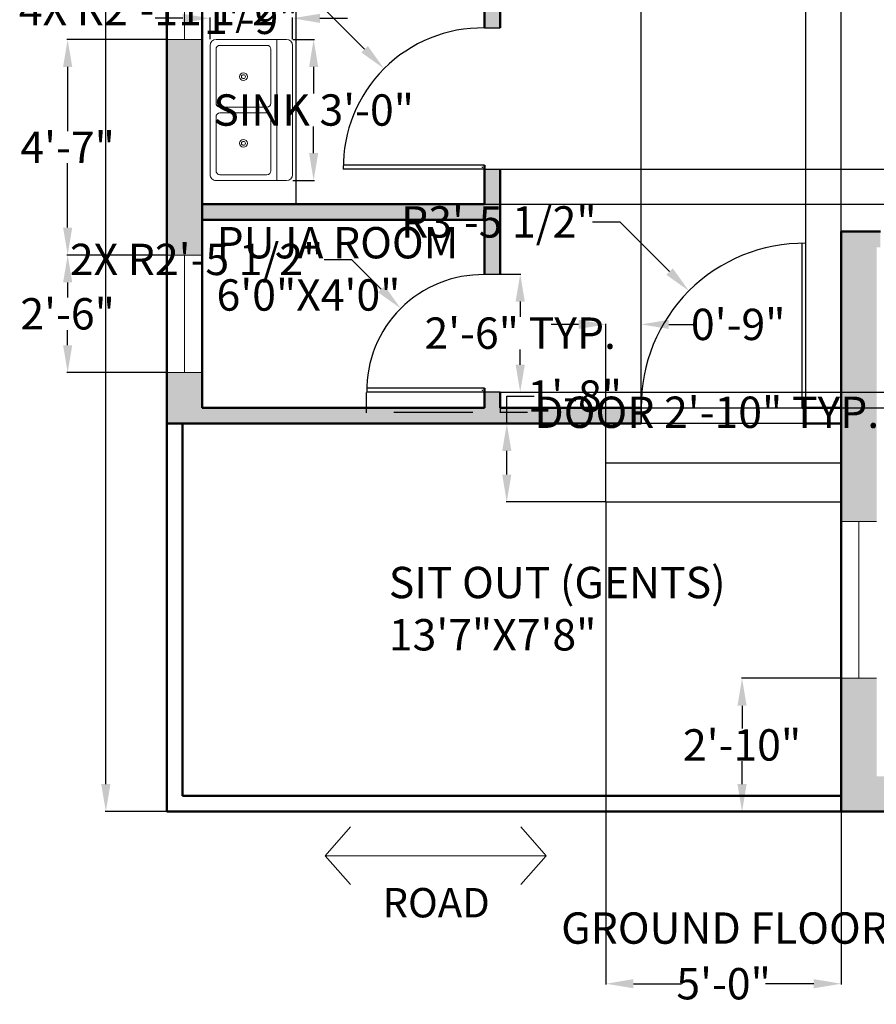
# Model space of a CAD drawing. Units: inches. Extents: x 808573 to 809030, y 884276 to 884799.
# Tile 1 of 4: x 808582 to 808801, y 884282 to 884534. Entities that reach past the tile are written whole.
import ezdxf

# ---------------------------------------------------------------- set-up
doc = ezdxf.new("R2010")
doc.units = ezdxf.units.IN
doc.header["$MEASUREMENT"] = 0
for name, color, linetype, lineweight in [('A-ANNO-DIMS', 2, 'Continuous', 18), ('A-ANNO-SYMB', 7, 'Continuous', 18), ('A-ANNO-TEXT', 7, 'Continuous', 25), ('A-AREA-IDEN', 7, 'Continuous', 25), ('A-DOOR', 3, 'Continuous', 25), ('A-FLOR-CASE', 9, 'Continuous', 25), ('A-FLOR-FIXT', 9, 'Continuous', 18), ('A-FLOR-STRS', 7, 'Continuous', 25), ('A-GLAZ', 4, 'Continuous', 18), ('A-WALL', 7, 'Continuous', 50)]:
    doc.layers.add(name, color=color, linetype=linetype, lineweight=lineweight)
doc.layers.add('A-WALL-PATT', color=251, linetype='Continuous', lineweight=13, true_color=0x636466)
doc.styles.get("Standard").update_dxf_attribs({"font": 'arial.ttf'})
doc.dimstyles.get("Standard").update_dxf_attribs({"dimtxt": 8, "dimasz": 7, "dimexe": 0.18, "dimexo": 0.0625, "dimgap": 0.09, "dimtad": 0, "dimtih": 1, "dimtoh": 1, "dimdec": 0, "dimzin": 0, "dimdsep": 46, "dimlunit": 3, "dimtxsty": 'Standard', "dimcen": 0.09, "dimadec": 0, "dimazin": 0, "dimtfac": 1, "dimtdec": 0, "dimtofl": 0, "dimtmove": 0, "dimatfit": 3, "dimfxl": 1, "dimtolj": 1, "dimtzin": 0, "dimarcsym": 0})

# ---------------------------------------------------------------- blocks, each defined once
blk = doc.blocks.new('Sink-double - 36 in top')
for p, q in [((-18, -4), (18, -4)), ((-0.75, -18.5), (-0.75, -6.5)), ((0.75, -6.5), (0.75, -18.5))]:
    blk.add_line(p, q)
for points in [[(-16.5, 0), (16.5, 0)], [(-18, -19.5), (-18, -1.5)], [(18, -1.5), (18, -19.5)], [(-16.5, -18.5), (-16.5, -6.5)], [(-15.5, -5.5), (-1.75, -5.5)], [(1.75, -5.5), (15.5, -5.5)], [(16.5, -6.5), (16.5, -18.5)], [(-1.75, -19.5), (-15.5, -19.5)], [(15.5, -19.5), (1.75, -19.5)], [(16.5, -21), (-16.5, -21)]]:
    blk.add_lwpolyline(points)
for centre, radius in [((-8.5, -12.5), 1), ((-8.5, -12.5), 0.5), ((8.5, -12.5), 1), ((8.5, -12.5), 0.5)]:
    blk.add_circle(centre, radius)
for centre, radius, start, end in [((-16.5, -1.5), 1.5, 90, 180), ((16.5, -1.5), 1.5, 0, 90), ((-15.5, -6.5), 1, 90, 180), ((-1.75, -6.5), 1, 0, 90), ((1.75, -6.5), 1, 90, 180), ((15.5, -6.5), 1, 0, 90), ((-16.5, -19.5), 1.5, 180, 270), ((-15.5, -18.5), 1, 180, 270), ((-1.75, -18.5), 1, 270, 0), ((1.75, -18.5), 1, 180, 270), ((15.5, -18.5), 1, 270, 0), ((16.5, -19.5), 1.5, 270, 0)]:
    blk.add_arc(centre, radius, start, end)
blk = doc.blocks.new('*D7')
at = {"layer": 'A-ANNO-DIMS', "color": 0, "lineweight": -2, "transparency": 16777216}
for p, q in [((808619.57, 884751.64), (808603.89, 884751.64)), ((808604.07, 884744.64), (808604.07, 884545.82)), ((808604.07, 884338.64), (808604.07, 884537.46)), ((808619.57, 884331.64), (808603.89, 884331.64))]:
    blk.add_line(p, q, dxfattribs=at)
at = {"layer": 'A-ANNO-DIMS', "color": 0, "transparency": 16777216}
for points in [[(808602.9, 884744.64), (808605.23, 884744.64), (808604.07, 884751.64)], [(808602.9, 884338.64), (808605.23, 884338.64), (808604.07, 884331.64)]]:
    blk.add_solid(points, dxfattribs=at)
at = {"layer": 'Defpoints', "color": 0, "transparency": 16777216}
for p in [(808619.63, 884751.64), (808604.07, 884331.64), (808619.63, 884331.64)]:
    blk.add_point(p, dxfattribs=at)
at = {"layer": 'A-ANNO-DIMS', "color": 0, "transparency": 16777216, "insert": (808604.07, 884541.64), "char_height": 8, "attachment_point": 5}
blk.add_mtext("\\A1;35'", dxfattribs=at)
blk = doc.blocks.new('DOOR-SWING-36IN')
for p, q in [((0, 0), (0, 36)), ((1, 0), (1, 36)), ((0, 0), (0, -4)), ((36, 0), (36, -4))]:
    blk.add_line(p, q)
blk.add_arc((0.5, 0.5), 35.5, 359.1931, 90.8069)
blk = doc.blocks.new('DOOR-SWING-30IN')
for p, q in [((0, 30), (-4, 30)), ((-4, 1), (-34, 1)), ((-4, 0), (-34, 0)), ((0, 0), (-4, 0))]:
    blk.add_line(p, q)
blk.add_arc((-4.5, 0.5), 29.5, 89.029, 180.971)
blk = doc.blocks.new('WIN-40IN')
for p, q in [((0, 0), (9, 0)), ((4.5, 0), (4.5, -40)), ((0, -40), (9, -40))]:
    blk.add_line(p, q)
blk = doc.blocks.new('WIN-36IN')
for p, q in [((0, 0), (-9, 0)), ((-4.5, 0), (-4.5, -36)), ((0, -36), (-9, -36))]:
    blk.add_line(p, q)
blk = doc.blocks.new('*D21')
at = {"layer": 'A-ANNO-DIMS', "color": 0, "lineweight": -2, "transparency": 16777216}
for p, q in [((808670.49, 884438.58), (808670.49, 884433.34)), ((808704.63, 884438.58), (808704.63, 884433.34)), ((808677.49, 884433.52), (808697.63, 884433.52)), ((808704.63, 884433.52), (808711.63, 884433.52))]:
    blk.add_line(p, q, dxfattribs=at)
at = {"layer": 'A-ANNO-DIMS', "color": 0, "transparency": 16777216}
for points in [[(808677.49, 884434.69), (808677.49, 884432.35), (808670.49, 884433.52)], [(808697.63, 884434.69), (808697.63, 884432.35), (808704.63, 884433.52)]]:
    blk.add_solid(points, dxfattribs=at)
at = {"layer": 'Defpoints', "color": 0, "transparency": 16777216}
for p in [(808670.49, 884438.64), (808704.63, 884438.64), (808704.63, 884433.52)]:
    blk.add_point(p, dxfattribs=at)
at = {"layer": 'A-ANNO-DIMS', "color": 0, "transparency": 16777216, "insert": (808757.33, 884433.52), "char_height": 8, "attachment_point": 5}
blk.add_mtext('\\A1;DOOR 2\'-10" TYP.', dxfattribs=at)
blk = doc.blocks.new('*D22')
at = {"layer": 'A-ANNO-DIMS', "color": 0, "lineweight": -2, "transparency": 16777216}
for p, q in [((808704.69, 884468.78), (808709.93, 884468.78)), ((808709.75, 884461.78), (808709.75, 884457.88)), ((808709.75, 884445.64), (808709.75, 884449.53)), ((808704.69, 884438.64), (808709.93, 884438.64))]:
    blk.add_line(p, q, dxfattribs=at)
at = {"layer": 'A-ANNO-DIMS', "color": 0, "transparency": 16777216}
for points in [[(808708.58, 884461.78), (808710.92, 884461.78), (808709.75, 884468.78)], [(808708.58, 884445.64), (808710.92, 884445.64), (808709.75, 884438.64)]]:
    blk.add_solid(points, dxfattribs=at)
at = {"layer": 'Defpoints', "color": 0, "transparency": 16777216}
for p in [(808704.63, 884468.78), (808709.75, 884468.78), (808704.63, 884438.64)]:
    blk.add_point(p, dxfattribs=at)
at = {"layer": 'A-ANNO-DIMS', "color": 0, "transparency": 16777216, "insert": (808709.75, 884453.71), "char_height": 8, "attachment_point": 5}
blk.add_mtext('\\A1;2\'-6" TYP.', dxfattribs=at)
blk = doc.blocks.new('*D31')
at = {"layer": 'A-ANNO-DIMS', "color": 0, "lineweight": -2, "transparency": 16777216}
for p, q in [((808651.73, 884528.64), (808657.25, 884528.64)), ((808657.07, 884521.64), (808657.07, 884514.87)), ((808657.07, 884499.64), (808657.07, 884506.41)), ((808651.73, 884492.64), (808657.25, 884492.64))]:
    blk.add_line(p, q, dxfattribs=at)
at = {"layer": 'A-ANNO-DIMS', "color": 0, "transparency": 16777216}
for points in [[(808655.9, 884521.64), (808658.23, 884521.64), (808657.07, 884528.64)], [(808655.9, 884499.64), (808658.23, 884499.64), (808657.07, 884492.64)]]:
    blk.add_solid(points, dxfattribs=at)
at = {"layer": 'Defpoints', "color": 0, "transparency": 16777216}
for p in [(808651.67, 884528.64), (808651.67, 884492.64), (808657.07, 884492.64)]:
    blk.add_point(p, dxfattribs=at)
at = {"layer": 'A-ANNO-DIMS', "color": 0, "transparency": 16777216, "insert": (808657.07, 884510.64), "char_height": 8, "attachment_point": 5}
blk.add_mtext('\\A1;SINK 3\'-0"', dxfattribs=at)
blk = doc.blocks.new('*D32')
at = {"layer": 'A-ANNO-DIMS', "color": 0, "lineweight": -2, "transparency": 16777216}
for p, q in [((808623.67, 884534.04), (808616.67, 884534.04)), ((808630.67, 884528.7), (808630.67, 884534.22)), ((808651.67, 884528.7), (808651.67, 884534.22)), ((808658.67, 884534.04), (808665.67, 884534.04))]:
    blk.add_line(p, q, dxfattribs=at)
at = {"layer": 'A-ANNO-DIMS', "color": 0, "transparency": 16777216}
for points in [[(808623.67, 884535.2), (808623.67, 884532.87), (808630.67, 884534.04)], [(808658.67, 884535.2), (808658.67, 884532.87), (808651.67, 884534.04)]]:
    blk.add_solid(points, dxfattribs=at)
at = {"layer": 'Defpoints', "color": 0, "transparency": 16777216}
for p in [(808651.67, 884534.04), (808630.67, 884528.64), (808651.67, 884528.64)]:
    blk.add_point(p, dxfattribs=at)
at = {"layer": 'A-ANNO-DIMS', "color": 0, "transparency": 16777216, "insert": (808641.17, 884534.04), "char_height": 8, "attachment_point": 5}
blk.add_mtext('\\A1;1\'-9"', dxfattribs=at)
blk = doc.blocks.new('*D33')
at = {"layer": 'A-ANNO-DIMS', "color": 0, "lineweight": -2, "transparency": 16777216}
for p, q in [((808619.57, 884473.64), (808594.15, 884473.64)), ((808594.33, 884466.64), (808594.33, 884462.81)), ((808594.33, 884450.64), (808594.33, 884454.47)), ((808619.57, 884443.64), (808594.15, 884443.64))]:
    blk.add_line(p, q, dxfattribs=at)
at = {"layer": 'A-ANNO-DIMS', "color": 0, "transparency": 16777216}
for points in [[(808593.16, 884466.64), (808595.5, 884466.64), (808594.33, 884473.64)], [(808593.16, 884450.64), (808595.5, 884450.64), (808594.33, 884443.64)]]:
    blk.add_solid(points, dxfattribs=at)
at = {"layer": 'Defpoints', "color": 0, "transparency": 16777216}
for p in [(808594.33, 884473.64), (808619.63, 884473.64), (808619.63, 884443.64)]:
    blk.add_point(p, dxfattribs=at)
at = {"layer": 'A-ANNO-DIMS', "color": 0, "transparency": 16777216, "insert": (808594.33, 884458.64), "char_height": 8, "attachment_point": 5}
blk.add_mtext('\\A1;2\'-6"', dxfattribs=at)
blk = doc.blocks.new('*D34')
at = {"layer": 'A-ANNO-DIMS', "color": 0, "lineweight": -2, "transparency": 16777216}
for p, q in [((808619.57, 884528.64), (808594.15, 884528.64)), ((808594.33, 884521.64), (808594.33, 884505.23)), ((808594.33, 884480.64), (808594.33, 884497.05)), ((808619.57, 884473.64), (808594.15, 884473.64))]:
    blk.add_line(p, q, dxfattribs=at)
at = {"layer": 'A-ANNO-DIMS', "color": 0, "transparency": 16777216}
for points in [[(808593.16, 884521.64), (808595.5, 884521.64), (808594.33, 884528.64)], [(808593.16, 884480.64), (808595.5, 884480.64), (808594.33, 884473.64)]]:
    blk.add_solid(points, dxfattribs=at)
at = {"layer": 'Defpoints', "color": 0, "transparency": 16777216}
for p in [(808594.33, 884528.64), (808619.63, 884528.64), (808619.63, 884473.64)]:
    blk.add_point(p, dxfattribs=at)
at = {"layer": 'A-ANNO-DIMS', "color": 0, "transparency": 16777216, "insert": (808594.33, 884501.14), "char_height": 8, "attachment_point": 5}
blk.add_mtext('\\A1;4\'-7"', dxfattribs=at)
blk = doc.blocks.new('*D40')
at = {"layer": 'A-ANNO-DIMS', "color": 0, "lineweight": -2, "transparency": 16777216}
for p, q in [((808619.63, 884331.7), (808619.63, 884777.12)), ((808626.63, 884776.94), (808692.17, 884776.94)), ((808784.63, 884776.94), (808719.08, 884776.94)), ((808791.63, 884331.7), (808791.63, 884777.12))]:
    blk.add_line(p, q, dxfattribs=at)
at = {"layer": 'A-ANNO-DIMS', "color": 0, "transparency": 16777216}
for points in [[(808626.63, 884778.11), (808626.63, 884775.77), (808619.63, 884776.94)], [(808784.63, 884778.11), (808784.63, 884775.77), (808791.63, 884776.94)]]:
    blk.add_solid(points, dxfattribs=at)
at = {"layer": 'Defpoints', "color": 0, "transparency": 16777216}
for p in [(808791.63, 884776.94), (808619.63, 884331.64), (808791.63, 884331.64)]:
    blk.add_point(p, dxfattribs=at)
at = {"layer": 'A-ANNO-DIMS', "color": 0, "transparency": 16777216, "insert": (808705.63, 884776.94), "char_height": 8, "attachment_point": 5}
blk.add_mtext('\\A1;14\'-4"', dxfattribs=at)
blk = doc.blocks.new('*D43')
at = {"layer": 'A-ANNO-DIMS', "color": 0, "lineweight": -2, "transparency": 16777216}
for p, q in [((808731.63, 884410.58), (808731.63, 884287.53)), ((808791.63, 884410.58), (808791.63, 884287.53)), ((808738.63, 884287.71), (808750.91, 884287.71)), ((808784.63, 884287.71), (808772.35, 884287.71))]:
    blk.add_line(p, q, dxfattribs=at)
at = {"layer": 'A-ANNO-DIMS', "color": 0, "transparency": 16777216}
for points in [[(808738.63, 884288.87), (808738.63, 884286.54), (808731.63, 884287.71)], [(808784.63, 884288.87), (808784.63, 884286.54), (808791.63, 884287.71)]]:
    blk.add_solid(points, dxfattribs=at)
at = {"layer": 'Defpoints', "color": 0, "transparency": 16777216}
for p in [(808731.63, 884410.64), (808791.63, 884410.64), (808791.63, 884287.71)]:
    blk.add_point(p, dxfattribs=at)
at = {"layer": 'A-ANNO-DIMS', "color": 0, "transparency": 16777216, "insert": (808761.63, 884287.71), "char_height": 8, "attachment_point": 5}
blk.add_mtext('\\A1;5\'-0"', dxfattribs=at)
blk = doc.blocks.new('*D44')
at = {"layer": 'A-ANNO-DIMS', "color": 0, "lineweight": -2, "transparency": 16777216}
for p, q in [((808706.33, 884430.64), (808706.33, 884437.64)), ((808706.33, 884437.64), (808713.33, 884437.64)), ((808731.57, 884430.64), (808706.15, 884430.64)), ((808706.33, 884417.64), (808706.33, 884423.64)), ((808731.57, 884410.64), (808706.15, 884410.64))]:
    blk.add_line(p, q, dxfattribs=at)
at = {"layer": 'A-ANNO-DIMS', "color": 0, "transparency": 16777216}
for points in [[(808705.16, 884423.64), (808707.5, 884423.64), (808706.33, 884430.64)], [(808705.16, 884417.64), (808707.5, 884417.64), (808706.33, 884410.64)]]:
    blk.add_solid(points, dxfattribs=at)
at = {"layer": 'Defpoints', "color": 0, "transparency": 16777216}
for p in [(808706.33, 884430.64), (808731.63, 884430.64), (808731.63, 884410.64)]:
    blk.add_point(p, dxfattribs=at)
at = {"layer": 'A-ANNO-DIMS', "color": 0, "transparency": 16777216, "insert": (808723.67, 884437.64), "char_height": 8, "attachment_point": 5}
blk.add_mtext('\\A1;1\'-8"', dxfattribs=at)
blk = doc.blocks.new('*D48')
at = {"layer": 'A-ANNO-DIMS', "color": 0, "lineweight": -2, "transparency": 16777216}
for p, q in [((808740.63, 884434.7), (808740.63, 884777.12)), ((808747.63, 884776.94), (808750.91, 884776.94)), ((808775.63, 884776.94), (808772.35, 884776.94)), ((808782.63, 884434.7), (808782.63, 884777.12))]:
    blk.add_line(p, q, dxfattribs=at)
at = {"layer": 'A-ANNO-DIMS', "color": 0, "transparency": 16777216}
for points in [[(808747.63, 884778.11), (808747.63, 884775.77), (808740.63, 884776.94)], [(808775.63, 884778.11), (808775.63, 884775.77), (808782.63, 884776.94)]]:
    blk.add_solid(points, dxfattribs=at)
at = {"layer": 'Defpoints', "color": 0, "transparency": 16777216}
for p in [(808782.63, 884776.94), (808740.63, 884434.64), (808782.63, 884434.64)]:
    blk.add_point(p, dxfattribs=at)
at = {"layer": 'A-ANNO-DIMS', "color": 0, "transparency": 16777216, "insert": (808761.63, 884776.94), "char_height": 8, "attachment_point": 5}
blk.add_mtext('\\A1;3\'-6"', dxfattribs=at)
blk = doc.blocks.new('*D50')
at = {"layer": 'A-ANNO-DIMS', "color": 0, "lineweight": -2, "transparency": 16777216}
for p, q in [((808724.63, 884455.94), (808717.63, 884455.94)), ((808731.63, 884430.7), (808731.63, 884456.12)), ((808740.63, 884430.7), (808740.63, 884456.12)), ((808747.63, 884455.94), (808754.63, 884455.94))]:
    blk.add_line(p, q, dxfattribs=at)
at = {"layer": 'A-ANNO-DIMS', "color": 0, "transparency": 16777216}
for points in [[(808724.63, 884457.11), (808724.63, 884454.77), (808731.63, 884455.94)], [(808747.63, 884457.11), (808747.63, 884454.77), (808740.63, 884455.94)]]:
    blk.add_solid(points, dxfattribs=at)
at = {"layer": 'Defpoints', "color": 0, "transparency": 16777216}
for p in [(808740.63, 884455.94), (808731.63, 884430.64), (808740.63, 884430.64)]:
    blk.add_point(p, dxfattribs=at)
at = {"layer": 'A-ANNO-DIMS', "color": 0, "transparency": 16777216, "insert": (808765.35, 884455.94), "char_height": 8, "attachment_point": 5}
blk.add_mtext('\\A1;0\'-9"', dxfattribs=at)
blk = doc.blocks.new('*D51')
at = {"layer": 'A-ANNO-DIMS', "color": 0, "lineweight": -2, "transparency": 16777216}
for p, q in [((808791.57, 884365.64), (808766.15, 884365.64)), ((808766.33, 884358.64), (808766.33, 884352.81)), ((808766.33, 884338.64), (808766.33, 884344.47)), ((808791.57, 884331.64), (808766.15, 884331.64))]:
    blk.add_line(p, q, dxfattribs=at)
at = {"layer": 'A-ANNO-DIMS', "color": 0, "transparency": 16777216}
for points in [[(808765.16, 884358.64), (808767.5, 884358.64), (808766.33, 884365.64)], [(808765.16, 884338.64), (808767.5, 884338.64), (808766.33, 884331.64)]]:
    blk.add_solid(points, dxfattribs=at)
at = {"layer": 'Defpoints', "color": 0, "transparency": 16777216}
for p in [(808766.33, 884365.64), (808791.63, 884365.64), (808791.63, 884331.64)]:
    blk.add_point(p, dxfattribs=at)
at = {"layer": 'A-ANNO-DIMS', "color": 0, "transparency": 16777216, "insert": (808766.33, 884348.64), "char_height": 8, "attachment_point": 5}
blk.add_mtext('\\A1;2\'-10"', dxfattribs=at)
blk = doc.blocks.new('*D53')
at = {"layer": 'A-ANNO-DIMS', "color": 0, "lineweight": -2, "transparency": 16777216}
for p, q in [((808992.93, 884502.59), (808992.93, 884509.59)), ((808700.69, 884495.59), (808993.11, 884495.59)), ((808700.69, 884486.64), (808993.11, 884486.64)), ((808992.93, 884479.64), (808992.93, 884472.64))]:
    blk.add_line(p, q, dxfattribs=at)
at = {"layer": 'A-ANNO-DIMS', "color": 0, "transparency": 16777216}
for points in [[(808991.76, 884502.59), (808994.1, 884502.59), (808992.93, 884495.59)], [(808991.76, 884479.64), (808994.1, 884479.64), (808992.93, 884486.64)]]:
    blk.add_solid(points, dxfattribs=at)
at = {"layer": 'Defpoints', "color": 0, "transparency": 16777216}
for p in [(808700.63, 884495.59), (808992.93, 884495.59), (808700.63, 884486.64)]:
    blk.add_point(p, dxfattribs=at)
at = {"layer": 'A-ANNO-DIMS', "color": 0, "transparency": 16777216, "insert": (808992.93, 884491.11), "char_height": 8, "attachment_point": 5}
blk.add_mtext('\\A1;0\'-9"', dxfattribs=at)
blk = doc.blocks.new('*D54')
at = {"layer": 'A-ANNO-DIMS', "color": 0, "lineweight": -2, "transparency": 16777216}
for p, q in [((808992.93, 884445.64), (808992.93, 884452.64)), ((808992.93, 884452.64), (808999.93, 884452.64)), ((808704.69, 884438.64), (808993.11, 884438.64)), ((808704.69, 884434.64), (808993.11, 884434.64)), ((808992.93, 884427.64), (808992.93, 884420.64))]:
    blk.add_line(p, q, dxfattribs=at)
at = {"layer": 'A-ANNO-DIMS', "color": 0, "transparency": 16777216}
for points in [[(808991.76, 884445.64), (808994.1, 884445.64), (808992.93, 884438.64)], [(808991.76, 884427.64), (808994.1, 884427.64), (808992.93, 884434.64)]]:
    blk.add_solid(points, dxfattribs=at)
at = {"layer": 'Defpoints', "color": 0, "transparency": 16777216}
for p in [(808704.63, 884438.64), (808992.93, 884438.64), (808704.63, 884434.64)]:
    blk.add_point(p, dxfattribs=at)
at = {"layer": 'A-ANNO-DIMS', "color": 0, "transparency": 16777216, "insert": (809010.65, 884452.64), "char_height": 8, "attachment_point": 5}
blk.add_mtext('\\A1;0\'-4"', dxfattribs=at)
blk = doc.blocks.new('*D55')
at = {"layer": 'A-ANNO-DIMS', "color": 0, "lineweight": -2, "transparency": 16777216}
for p, q in [((808728.17, 884482.09), (808735.17, 884482.09)), ((808735.17, 884482.09), (808747.83, 884469.44)), ((808782.04, 884435.14), (808782.22, 884435.14)), ((808782.13, 884435.05), (808782.13, 884435.23))]:
    blk.add_line(p, q, dxfattribs=at)
at = {"layer": 'A-ANNO-DIMS', "color": 0, "transparency": 16777216}
blk.add_solid([(808748.66, 884470.26), (808747.01, 884468.61), (808752.78, 884464.49)], dxfattribs=at)
at = {"layer": 'Defpoints', "color": 0, "transparency": 16777216}
for p in [(808752.78, 884464.49), (808782.13, 884435.14)]:
    blk.add_point(p, dxfattribs=at)
at = {"layer": 'A-ANNO-DIMS', "color": 0, "transparency": 16777216, "insert": (808704.3, 884482.09), "char_height": 8, "attachment_point": 5}
blk.add_mtext('\\A1;R3\'-5 1/2"', dxfattribs=at)
blk = doc.blocks.new('*D56')
at = {"layer": 'A-ANNO-DIMS', "color": 0, "lineweight": -2, "transparency": 16777216}
for p, q in [((808652.96, 884536.26), (808659.96, 884536.26)), ((808659.96, 884536.26), (808670.07, 884526.14)), ((808700.04, 884496.09), (808700.22, 884496.09)), ((808700.13, 884496), (808700.13, 884496.18))]:
    blk.add_line(p, q, dxfattribs=at)
at = {"layer": 'A-ANNO-DIMS', "color": 0, "transparency": 16777216}
blk.add_solid([(808670.9, 884526.97), (808669.25, 884525.32), (808675.02, 884521.19)], dxfattribs=at)
at = {"layer": 'Defpoints', "color": 0, "transparency": 16777216}
for p in [(808675.02, 884521.19), (808700.13, 884496.09)]:
    blk.add_point(p, dxfattribs=at)
at = {"layer": 'A-ANNO-DIMS', "color": 0, "transparency": 16777216, "insert": (808617.23, 884536.26), "char_height": 8, "attachment_point": 5}
blk.add_mtext('\\A1;4X R2\'-11 1/2"', dxfattribs=at)
blk = doc.blocks.new('*D57')
at = {"layer": 'A-ANNO-DIMS', "color": 0, "lineweight": -2, "transparency": 16777216}
for p, q in [((808659.75, 884472.52), (808666.75, 884472.52)), ((808666.75, 884472.52), (808674.32, 884464.95)), ((808700.04, 884439.14), (808700.22, 884439.14)), ((808700.13, 884439.05), (808700.13, 884439.23))]:
    blk.add_line(p, q, dxfattribs=at)
at = {"layer": 'A-ANNO-DIMS', "color": 0, "transparency": 16777216}
blk.add_solid([(808675.14, 884465.78), (808673.49, 884464.13), (808679.27, 884460)], dxfattribs=at)
at = {"layer": 'Defpoints', "color": 0, "transparency": 16777216}
for p in [(808679.27, 884460), (808700.13, 884439.14)]:
    blk.add_point(p, dxfattribs=at)
at = {"layer": 'A-ANNO-DIMS', "color": 0, "transparency": 16777216, "insert": (808627.21, 884472.52), "char_height": 8, "attachment_point": 5}
blk.add_mtext('\\A1;2X R2\'-5 1/2"', dxfattribs=at)

msp = doc.modelspace()

# ---------------------------------------------------------------- hatches: boundary and pattern name
at = {"layer": 'A-WALL-PATT'}
h = msp.add_hatch(color=256, dxfattribs=at)
h.dxf.hatch_style = 1
h.paths.add_polyline_path([(808967.63, 884751.64), (808619.63, 884751.64), (808619.63, 884696.64), (808628.63, 884696.64), (808628.63, 884742.64), (808791.63, 884742.64), (808958.63, 884742.64), (808958.63, 884696.64), (808967.63, 884696.64)])
h.paths.add_polyline_path([(808967.63, 884656.64), (808958.63, 884656.64), (808958.63, 884610.64), (808958.63, 884590.14), (808967.63, 884590.14)])
h.paths.add_polyline_path([(808967.63, 884494.64), (808958.63, 884494.64), (808958.63, 884479.64), (808958.63, 884340.64), (808901.23, 884340.64), (808901.23, 884331.64), (808967.63, 884331.64)])
h.paths.add_polyline_path([(808967.63, 884554.14), (808958.63, 884554.14), (808958.63, 884537.64), (808875.63, 884537.64), (808875.63, 884533.64), (808884.63, 884533.64), (808884.63, 884479.64), (808841.63, 884479.64), (808841.63, 884533.64), (808845.63, 884533.64), (808845.63, 884537.64), (808837.63, 884537.64), (808837.63, 884479.64), (808837.63, 884475.64), (808958.63, 884475.64), (808958.63, 884479.64), (808888.63, 884479.64), (808888.63, 884533.64), (808958.63, 884533.64), (808958.63, 884518.64), (808967.63, 884518.64)])
h.paths.add_polyline_path([(808858.03, 884340.64), (808800.63, 884340.64), (808800.63, 884365.64), (808791.63, 884365.64), (808791.63, 884331.64), (808858.03, 884331.64)])
h.paths.add_polyline_path([(808800.63, 884475.64), (808801.63, 884475.64), (808801.63, 884479.64), (808791.63, 884479.64), (808791.63, 884430.64), (808791.63, 884405.64), (808800.63, 884405.64)])
h.paths.add_polyline_path([(808740.63, 884434.64), (808704.63, 884434.64), (808704.63, 884438.64), (808700.63, 884438.64), (808700.63, 884434.64), (808628.63, 884434.64), (808628.63, 884443.64), (808619.63, 884443.64), (808619.63, 884430.64), (808740.63, 884430.64)])
h.paths.add_polyline_path([(808628.63, 884528.64), (808619.63, 884528.64), (808619.63, 884473.64), (808628.63, 884473.64), (808628.63, 884482.64)])
h.paths.add_polyline_path([(808628.63, 884606.64), (808628.63, 884656.64), (808619.63, 884656.64), (808619.63, 884564.64), (808628.63, 884564.64)])
h.paths.add_polyline_path([(808704.63, 884482.64), (808704.63, 884495.59), (808700.63, 884495.59), (808700.63, 884486.64), (808628.63, 884486.64), (808628.63, 884482.64), (808700.63, 884482.64), (808700.63, 884468.64), (808704.63, 884468.64)])
h.paths.add_polyline_path([(808704.63, 884606.64), (808700.63, 884606.64), (808700.63, 884531.59), (808704.63, 884531.59)])
h.paths.add_polyline_path([(808746.63, 884610.64), (808628.63, 884610.64), (808628.63, 884606.64), (808746.63, 884606.64)])
h.paths.add_polyline_path([(808804.63, 884610.64), (808795.63, 884610.64), (808795.63, 884742.64), (808791.63, 884742.64), (808791.63, 884610.64), (808782.63, 884610.64), (808782.63, 884606.64), (808804.63, 884606.64)])
h.paths.add_polyline_path([(808958.63, 884610.64), (808840.63, 884610.64), (808840.63, 884606.64), (808958.63, 884606.64)])

# ---------------------------------------------------------------- linework, layer by layer
at = {"layer": 'A-ANNO-SYMB'}
for p, q in [((808660, 884320.37), (808666.48, 884327.74)), ((808716.37, 884320.37), (808709.88, 884327.74)), ((808660, 884320.37), (808716.37, 884320.37)), ((808660, 884320.37), (808666.48, 884313.01)), ((808716.37, 884320.37), (808709.88, 884313.01))]:
    msp.add_line(p, q, dxfattribs=at)
at = {"layer": 'A-DOOR'}
for p, q in [((808781.63, 884434.64), (808781.63, 884476.64)), ((808782.63, 884434.64), (808782.63, 884476.64)), ((808740.63, 884434.64), (808740.63, 884430.64)), ((808782.63, 884434.64), (808782.63, 884430.64))]:
    msp.add_line(p, q, dxfattribs=at)
msp.add_arc((808782.13, 884435.14), 41.5, 89.3097, 180.6903, dxfattribs=at)
at = {"layer": 'A-FLOR-CASE'}
msp.add_line((808652.63, 884486.64), (808652.63, 884582.64), dxfattribs=at)
at = {"layer": 'A-FLOR-STRS'}
for p, q in [((808731.63, 884410.64), (808731.63, 884430.64)), ((808782.63, 884430.64), (808740.63, 884430.64)), ((808731.63, 884420.64), (808791.63, 884420.64)), ((808731.63, 884410.64), (808791.63, 884410.64))]:
    msp.add_line(p, q, dxfattribs=at)
at = {"layer": 'A-GLAZ'}
for p, q in [((808628.63, 884473.64), (808619.63, 884473.64)), ((808624.13, 884473.64), (808624.13, 884443.64)), ((808628.63, 884443.64), (808619.63, 884443.64))]:
    msp.add_line(p, q, dxfattribs=at)
at = {"layer": 'A-WALL'}
for p, q in [((808619.63, 884331.64), (808619.63, 884751.64)), ((808628.63, 884482.64), (808628.63, 884606.64)), ((808700.63, 884531.59), (808700.63, 884606.64)), ((808704.63, 884531.59), (808704.63, 884606.64)), ((808700.63, 884486.64), (808700.63, 884496.59)), ((808704.63, 884482.64), (808704.63, 884495.59)), ((808628.63, 884486.64), (808700.63, 884486.64)), ((808628.63, 884482.64), (808700.63, 884482.64)), ((808628.63, 884434.64), (808628.63, 884482.64)), ((808700.63, 884468.64), (808700.63, 884482.64)), ((808704.63, 884468.64), (808704.63, 884482.64)), ((808791.63, 884430.64), (808791.63, 884479.64)), ((808801.63, 884479.64), (808791.63, 884479.64)), ((808700.63, 884434.64), (808700.63, 884439.64)), ((808704.63, 884434.64), (808704.63, 884438.64)), ((808628.63, 884434.64), (808700.63, 884434.64)), ((808628.63, 884434.64), (808700.63, 884434.64)), ((808704.63, 884434.64), (808740.63, 884434.64)), ((808781.63, 884434.64), (808791.63, 884434.64)), ((808619.63, 884430.64), (808740.63, 884430.64)), ((808623.63, 884335.64), (808623.63, 884430.64)), ((808782.63, 884430.64), (808791.63, 884430.64)), ((808791.63, 884331.64), (808791.63, 884430.64)), ((808623.63, 884335.64), (808791.63, 884335.64)), ((808967.63, 884331.64), (808619.63, 884331.64))]:
    msp.add_line(p, q, dxfattribs=at)

# ---------------------------------------------------------------- block references
at = {"layer": 'A-DOOR', "rotation": 89.99999999989896}
msp.add_blockref('DOOR-SWING-36IN', (808700.63, 884495.59), dxfattribs=at)
at = {"layer": 'A-DOOR'}
msp.add_blockref('DOOR-SWING-30IN', (808704.63, 884438.64), dxfattribs=at)
at = {"layer": 'A-FLOR-FIXT', "rotation": 270}
msp.add_blockref('Sink-double - 36 in top', (808651.67, 884510.64), dxfattribs=at)
at = {"layer": 'A-GLAZ'}
for name, p in [('WIN-36IN', (808628.63, 884564.64)), ('WIN-40IN', (808791.63, 884405.64))]:
    msp.add_blockref(name, p, dxfattribs=at)

# ---------------------------------------------------------------- texts
at = {"layer": 'A-ANNO-TEXT', "attachment_point": 1}
for s, width, insert, char_height in [('ROAD', 27.9171, (808674.64, 884312.13), 7.5), ('{\\fArial|b1|i0|c0|p34;GROUND FLOOR PLAN}', 273.1721, (808720.2, 884305.91), 8)]:
    msp.add_mtext_dynamic_manual_height_columns(s, width=width, gutter_width=1, heights=[0], dxfattribs=dict(at, insert=insert, char_height=char_height))
at = {"layer": 'A-AREA-IDEN', "char_height": 8, "attachment_point": 1}
for s, insert in [('PUJA ROOM\\P6\'0"X4\'0"', (808632.31, 884480.78)), ('SIT OUT (GENTS)\\P13\'7"X7\'8"', (808676.24, 884394.08))]:
    msp.add_mtext_dynamic_manual_height_columns(s, width=94.1107, gutter_width=1, heights=[0], dxfattribs=dict(at, insert=insert))

# ---------------------------------------------------------------- dimensions: what is measured, and where the dimension line sits
at = {"layer": 'A-ANNO-DIMS'}
for base, p1, p2, picture, middle in [((808791.63, 884776.94), (808619.63, 884331.64), (808791.63, 884331.64), '*D40', (808705.63, 884776.94)), ((808782.63, 884776.94), (808740.63, 884434.64), (808782.63, 884434.64), '*D48', (808761.63, 884776.94)), ((808651.67, 884534.04), (808630.67, 884528.64), (808651.67, 884528.64), '*D32', (808641.17, 884534.04)), ((808740.63, 884455.94), (808731.63, 884430.64), (808740.63, 884430.64), '*D50', (808765.35, 884455.94)), ((808791.63, 884287.71), (808731.63, 884410.64), (808791.63, 884410.64), '*D43', (808761.63, 884287.71))]:
    dim = msp.add_linear_dim(base=base, p1=p1, p2=p2, dimstyle='Standard', override={"dimdec": 1, "dimlfac": 1, "dimrnd": 0, "dimzin": 1, "dimdsep": 46, "dimlunit": 4, "dimfrac": 2}, dxfattribs=at)
    dim.commit()
    dim.dimension.update_dxf_attribs({"geometry": picture, "text_midpoint": middle})
for base, p1, p2, override, picture, middle in [((808604.07, 884331.64), (808619.63, 884751.64), (808619.63, 884331.64), {"dimclrd": 0, "dimclre": 0, "dimclrt": 0}, '*D7', (808604.07, 884541.64)), ((808594.33, 884528.64), (808619.63, 884473.64), (808619.63, 884528.64), {"dimdec": 1, "dimlfac": 1, "dimrnd": 0, "dimzin": 1, "dimdsep": 46, "dimlunit": 4, "dimfrac": 2}, '*D34', (808594.33, 884501.14)), ((808992.9284, 884495.5872), (808700.6284, 884486.64), (808700.6284, 884495.5872), {"dimdec": 1, "dimlfac": 1, "dimrnd": 0, "dimzin": 1, "dimdsep": 46, "dimlunit": 4, "dimfrac": 2}, '*D53', (808992.9284, 884491.1136)), ((808594.33, 884473.64), (808619.63, 884443.64), (808619.63, 884473.64), {"dimdec": 1, "dimlfac": 1, "dimrnd": 0, "dimzin": 1, "dimdsep": 46, "dimlunit": 4, "dimfrac": 2}, '*D33', (808594.33, 884458.64)), ((808992.93, 884438.64), (808704.63, 884434.64), (808704.63, 884438.64), {"dimdec": 1, "dimlfac": 1, "dimrnd": 0, "dimzin": 1, "dimdsep": 46, "dimlunit": 4, "dimfrac": 2}, '*D54', (809010.65, 884452.64)), ((808706.33, 884430.64), (808731.63, 884410.64), (808731.63, 884430.64), {"dimdec": 1, "dimlfac": 1, "dimrnd": 0, "dimzin": 1, "dimdsep": 46, "dimlunit": 4, "dimfrac": 2}, '*D44', (808723.67, 884437.64)), ((808766.33, 884365.64), (808791.63, 884331.64), (808791.63, 884365.64), {"dimdec": 1, "dimlfac": 1, "dimrnd": 0, "dimzin": 1, "dimdsep": 46, "dimlunit": 4, "dimfrac": 2}, '*D51', (808766.33, 884348.64))]:
    dim = msp.add_linear_dim(base=base, p1=p1, p2=p2, angle=90, dimstyle='Standard', override=override, dxfattribs=at)
    dim.commit()
    dim.dimension.update_dxf_attribs({"geometry": picture, "text_midpoint": middle})
for center, mpoint, text, picture, middle in [((808700.13, 884496.09), (808675.02, 884521.19), '4X <>', '*D56', (808617.23, 884536.26)), ((808700.13, 884439.14), (808679.27, 884460), '2X <>', '*D57', (808627.21, 884472.52))]:
    dim = msp.add_radius_dim(center=center, mpoint=mpoint, text=text, dimstyle='Standard', override={"dimdec": 1, "dimlfac": 1, "dimrnd": 0, "dimzin": 1, "dimdsep": 46, "dimlunit": 4, "dimfrac": 2}, dxfattribs=at)
    dim.commit()
    dim.dimension.update_dxf_attribs({"geometry": picture, "text_midpoint": middle, "dimtype": 164})
for base, p1, p2, angle, text, picture, middle in [((808657.07, 884492.64), (808651.67, 884528.64), (808651.67, 884492.64), 270, 'SINK <>', '*D31', (808657.07, 884510.64)), ((808709.75, 884468.78), (808704.63, 884438.64), (808704.63, 884468.78), 90, '<> TYP.', '*D22', (808709.75, 884453.71))]:
    dim = msp.add_linear_dim(base=base, p1=p1, p2=p2, angle=angle, text=text, dimstyle='Standard', override={"dimdec": 1, "dimlfac": 1, "dimrnd": 0, "dimzin": 1, "dimdsep": 46, "dimlunit": 4, "dimfrac": 2}, dxfattribs=at)
    dim.commit()
    dim.dimension.update_dxf_attribs({"geometry": picture, "text_midpoint": middle})
dim = msp.add_radius_dim(center=(808782.13, 884435.14), mpoint=(808752.78, 884464.49), dimstyle='Standard', override={"dimdec": 1, "dimlfac": 1, "dimrnd": 0, "dimzin": 1, "dimdsep": 46, "dimlunit": 4, "dimfrac": 2}, dxfattribs=at)
dim.commit()
dim.dimension.update_dxf_attribs({"geometry": '*D55', "text_midpoint": (808704.3, 884482.09), "dimtype": 164})
dim = msp.add_linear_dim(base=(808704.63, 884433.52), p1=(808670.49, 884438.64), p2=(808704.63, 884438.64), text='DOOR <> TYP.', dimstyle='Standard', override={"dimdec": 1, "dimlfac": 1, "dimrnd": 0, "dimzin": 1, "dimdsep": 46, "dimlunit": 4, "dimfrac": 2}, dxfattribs=at)
dim.commit()
dim.dimension.update_dxf_attribs({"geometry": '*D21', "text_midpoint": (808757.33, 884433.52)})

doc.saveas('drawing.dxf')
